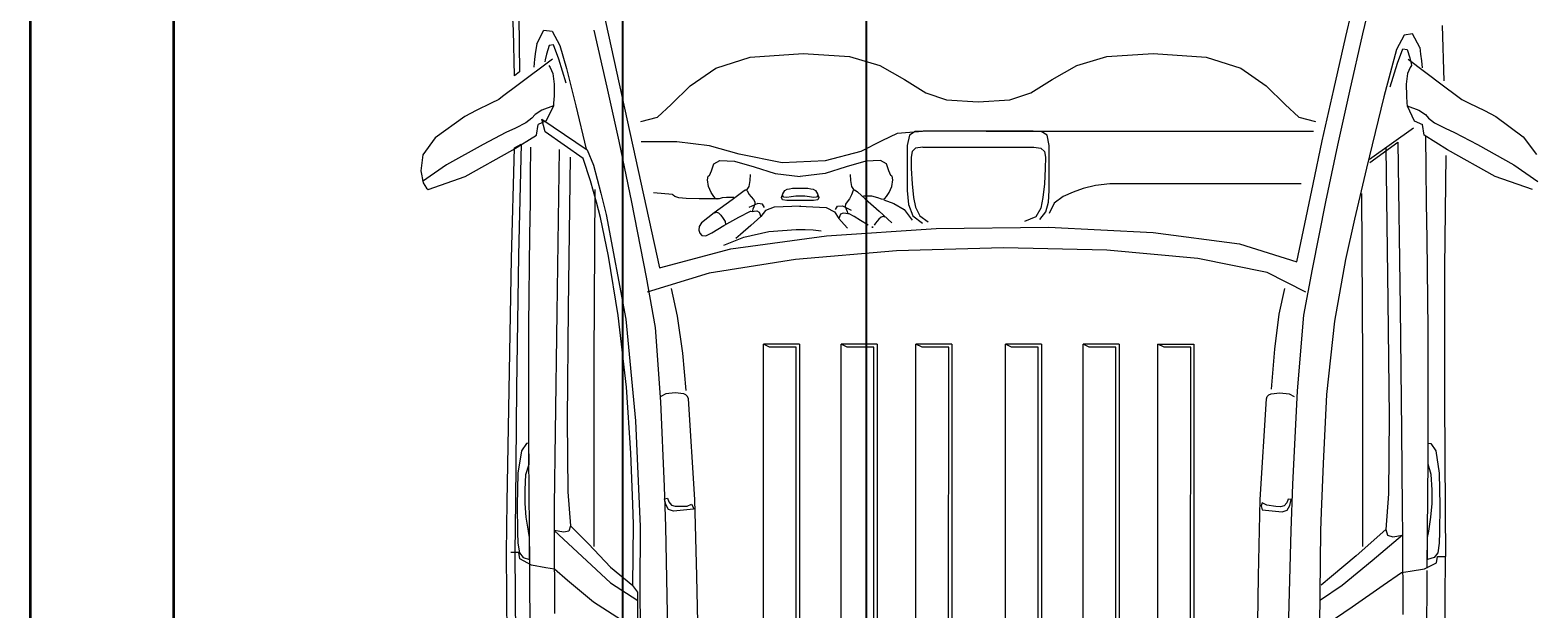
# Model space of a CAD drawing. Units: inches. Extents: x 5 to 421, y -617 to 43.
# Tile 3 of 15: x 37 to 132, y -505 to -469. Entities that reach past the tile are written whole.
import ezdxf

# ---------------------------------------------------------------- set-up
doc = ezdxf.new("R2010")
doc.units = ezdxf.units.IN
doc.header["$MEASUREMENT"] = 0
for name, color, linetype, lineweight in [('A-ANNO-DIMS', 2, 'Continuous', 18), ('A-SITE-VEHC', 8, 'Continuous', 13), ('A-WALL', 7, 'Continuous', 35)]:
    doc.layers.add(name, color=color, linetype=linetype, lineweight=lineweight)
doc.styles.get("Standard").update_dxf_attribs({"font": 'arial.ttf'})
doc.dimstyles.get("Standard").update_dxf_attribs({"dimtxt": 0.18, "dimasz": 0.18, "dimexe": 0.18, "dimexo": 0.0625, "dimgap": 0.09, "dimtad": 0, "dimtih": 1, "dimtoh": 1, "dimdec": 0, "dimzin": 0, "dimdsep": 46, "dimlunit": 3, "dimtxsty": 'Standard', "dimcen": 0.09, "dimadec": 0, "dimazin": 0, "dimtfac": 1, "dimtdec": 0, "dimtofl": 0, "dimtmove": 0, "dimatfit": 3, "dimfxl": 1, "dimtolj": 1, "dimtzin": 0, "dimarcsym": 0})

# ---------------------------------------------------------------- blocks, each defined once
blk = doc.blocks.new('*D78')
at = {"layer": 'A-ANNO-DIMS', "color": 0, "lineweight": -2, "transparency": 16777216}
for p, q in [((74.624, -338.19), (74.624, -616.599)), ((89.924, -338.331), (89.924, -616.599)), ((74.804, -616.419), (81.958, -616.419)), ((89.744, -616.419), (82.589, -616.419))]:
    blk.add_line(p, q, dxfattribs=at)
at = {"layer": 'A-ANNO-DIMS', "color": 0, "transparency": 16777216}
for points in [[(74.804, -616.389), (74.804, -616.449), (74.624, -616.419)], [(89.744, -616.389), (89.744, -616.449), (89.924, -616.419)]]:
    blk.add_solid(points, dxfattribs=at)
at = {"layer": 'Defpoints', "color": 0, "transparency": 16777216}
for p in [(74.624, -338.127), (89.924, -338.269), (89.924, -616.419)]:
    blk.add_point(p, dxfattribs=at)
at = {"layer": 'A-ANNO-DIMS', "color": 0, "transparency": 16777216, "insert": (82.274, -616.419), "char_height": 0.18, "attachment_point": 5}
blk.add_mtext('\\A1;15.3', dxfattribs=at)

msp = doc.modelspace()

# ---------------------------------------------------------------- linework, layer by layer
at = {"layer": 'A-SITE-VEHC'}
for p, q in [((67.7642, -468.9053), (67.6725, -466.951)), ((73.4116, -467.6765), (76.9484, -483.8294)), ((121.4807, -467.4597), (121.0957, -469.1284)), ((68.1156, -468.0292), (68.1428, -471.5036)), ((120.0545, -469.2979), (120.4101, -467.7799)), ((126.0856, -468.6013), (126.1926, -472.0787)), ((67.8382, -471.7647), (67.7642, -468.9053)), ((69.2294, -469.7473), (69.6829, -468.8901)), ((69.6829, -468.8901), (70.1988, -468.9567)), ((70.1988, -468.9567), (70.69, -469.8597)), ((72.8166, -468.888), (73.6384, -472.4794)), ((119.2871, -472.6093), (120.0545, -469.2979)), ((121.0957, -469.1284), (120.2738, -472.7197)), ((123.7131, -469.197), (123.2221, -470.1)), ((124.2292, -469.1304), (123.7131, -469.197)), ((124.6827, -469.9876), (124.2292, -469.1304)), ((69.1614, -470.2267), (69.1022, -470.7152)), ((69.2294, -469.7473), (69.1614, -470.2267)), ((69.843, -470.3966), (69.7577, -470.7462)), ((70.0157, -469.8597), (69.843, -470.3966)), ((70.28, -469.8223), (70.0157, -469.8597)), ((70.6316, -470.7212), (70.28, -469.8223)), ((70.69, -469.8597), (71.0943, -471.2901)), ((82.6431, -470.5843), (85.9655, -470.3515)), ((85.9655, -470.3515), (88.8787, -470.5475)), ((88.8787, -470.5475), (90.7773, -471.1094)), ((103.1439, -471.1094), (105.0426, -470.5475)), ((105.0426, -470.5475), (107.9558, -470.3515)), ((107.9558, -470.3515), (111.2783, -470.5843)), ((123.2221, -470.1), (122.4253, -473.0796)), ((123.2804, -470.9615), (123.632, -470.0626)), ((123.632, -470.0626), (123.8964, -470.1)), ((123.8964, -470.1), (124.069, -470.6368)), ((124.6827, -469.9876), (124.7423, -470.4038)), ((124.7423, -470.4038), (124.7953, -470.8268)), ((68.1428, -471.5036), (67.8382, -471.7647)), ((70.2201, -470.718), (68.0729, -472.3222)), ((69.1022, -470.7152), (69.0508, -471.213)), ((69.7577, -470.7462), (69.7349, -470.8711)), ((69.9956, -471.1111), (70.083, -471.2298)), ((70.083, -471.2298), (70.2453, -471.6105)), ((71.0831, -472.2194), (70.6316, -470.7212)), ((71.0943, -471.2901), (71.6877, -473.6545)), ((78.8717, -472.3887), (80.4797, -471.2698)), ((80.4797, -471.2698), (82.6431, -470.5843)), ((90.7773, -471.1094), (92.3227, -471.9987)), ((101.5986, -471.9987), (103.1439, -471.1094)), ((111.2783, -470.5843), (113.4418, -471.2698)), ((113.4418, -471.2698), (115.0496, -472.3887)), ((122.8289, -472.4594), (123.2804, -470.9615)), ((124.0898, -471.2298), (123.9277, -471.6105)), ((123.9524, -470.718), (126.0997, -472.3222)), ((124.069, -470.6368), (124.1543, -470.9863)), ((124.1771, -471.1111), (124.0898, -471.2298)), ((124.1543, -470.9863), (124.1771, -471.1111)), ((124.7953, -470.8268), (124.8422, -471.2569)), ((68.0729, -472.3222), (67.0866, -473.065)), ((70.2453, -471.6105), (70.3327, -472.291)), ((70.3327, -472.291), (70.3182, -473.015)), ((77.6783, -473.5667), (78.8717, -472.3887)), ((92.3227, -471.9987), (93.6601, -472.8207)), ((100.2614, -472.8207), (101.5986, -471.9987)), ((115.0496, -472.3887), (116.2431, -473.5667)), ((123.9277, -471.6105), (123.8403, -472.291)), ((123.8403, -472.291), (123.8549, -473.015)), ((126.0997, -472.3222), (127.086, -473.065)), ((66.8494, -473.2461), (66.373, -473.4764)), ((67.0866, -473.065), (66.8494, -473.2461)), ((70.3182, -473.015), (70.291, -473.4769)), ((73.6384, -472.4794), (74.3978, -475.8708)), ((93.6601, -472.8207), (94.9685, -473.2574)), ((94.9685, -473.2574), (96.9608, -473.3858)), ((96.9608, -473.3858), (98.953, -473.2574)), ((98.953, -473.2574), (100.2614, -472.8207)), ((118.5569, -475.8501), (119.2871, -472.6093)), ((120.2738, -472.7197), (119.5142, -476.1112)), ((122.4253, -473.0796), (121.3413, -477.5698)), ((123.8549, -473.015), (123.8818, -473.4769)), ((127.086, -473.065), (127.3231, -473.2461)), ((127.3231, -473.2461), (127.7999, -473.4756)), ((64.7148, -474.3134), (62.8626, -475.6479)), ((65.4224, -473.9441), (64.7148, -474.3134)), ((66.373, -473.4764), (65.4224, -473.9441)), ((69.1278, -474.1845), (68.9282, -474.4258)), ((69.5523, -473.9181), (69.1278, -474.1845)), ((70.2764, -473.6392), (69.5523, -473.9181)), ((70.2764, -473.6392), (69.8269, -474.5943)), ((70.291, -473.4769), (70.2764, -473.6392)), ((71.6877, -473.6545), (72.3416, -476.3662)), ((75.7798, -474.6283), (76.8189, -474.356)), ((76.8189, -474.356), (77.6783, -473.5667)), ((116.2431, -473.5667), (117.1025, -474.356)), ((117.1025, -474.356), (118.1418, -474.6283)), ((123.8818, -473.4769), (123.8964, -473.6392)), ((123.8964, -473.6392), (124.3459, -474.5943)), ((123.8964, -473.6392), (124.6203, -473.9181)), ((124.6203, -473.9181), (125.0448, -474.1845)), ((125.0448, -474.1845), (125.2446, -474.4258)), ((127.7999, -473.4756), (128.7512, -473.9425)), ((128.7512, -473.9425), (129.458, -474.3134)), ((129.458, -474.3134), (131.1824, -475.5849)), ((67.8961, -475.0418), (67.2989, -475.3245)), ((68.5557, -474.7088), (67.8961, -475.0418)), ((68.9282, -474.4258), (68.5557, -474.7088)), ((69.209, -475.4933), (69.3213, -474.819)), ((69.8269, -474.5943), (69.3213, -474.819)), ((69.5573, -474.4845), (72.4075, -476.3993)), ((69.753, -475.2679), (69.5573, -474.4845)), ((72.1464, -476.9434), (69.753, -475.2679)), ((93.732, -475.2351), (91.865, -475.3861)), ((93.0014, -475.264), (92.6364, -475.4898)), ((93.5076, -475.2374), (93.0014, -475.264)), ((100.414, -475.2374), (93.5076, -475.2374)), ((97.4687, -475.2546), (93.732, -475.2351)), ((103.1448, -475.2665), (97.4687, -475.2546)), ((100.9201, -475.264), (100.414, -475.2374)), ((101.2849, -475.4898), (100.9201, -475.264)), ((110.1834, -475.2654), (103.1448, -475.2665)), ((118.0075, -475.2463), (110.1834, -475.2654)), ((124.2895, -475.0438), (121.5368, -477.0099)), ((124.3459, -474.5943), (124.8514, -474.819)), ((124.9638, -475.4933), (124.8514, -474.819)), ((125.2446, -474.4258), (125.617, -474.7088)), ((125.617, -474.7088), (126.2767, -475.0418)), ((126.2767, -475.0418), (126.874, -475.3245)), ((62.8626, -475.6479), (62.0839, -476.7266)), ((65.8678, -476.071), (63.574, -477.3502)), ((67.2989, -475.3245), (65.8678, -476.071)), ((67.7321, -476.4144), (69.209, -475.4933)), ((67.8382, -476.2907), (68.2514, -476.0431)), ((68.2514, -476.0431), (68.0884, -483.0214)), ((68.8353, -476.2417), (68.8173, -478.0422)), ((74.3978, -475.8708), (75.191, -479.7057)), ((78.036, -475.8989), (75.7823, -475.8989)), ((80.0909, -476.16), (78.036, -475.8989)), ((81.9383, -476.6824), (80.0909, -476.16)), ((90.9118, -475.8357), (89.5976, -476.5082)), ((91.865, -475.3861), (90.9118, -475.8357)), ((92.6364, -475.4898), (92.4962, -476.1328)), ((92.4962, -476.1328), (92.4962, -478.9649)), ((93.4786, -476.2485), (93.0243, -476.3068)), ((93.4786, -476.2485), (100.4427, -476.2485)), ((100.4427, -476.2485), (100.897, -476.3068)), ((101.4251, -476.1328), (101.2849, -475.4898)), ((101.4251, -478.9649), (101.4251, -476.1328)), ((117.9842, -478.5661), (118.5569, -475.8501)), ((119.5142, -476.1112), (118.7684, -479.682)), ((121.5478, -477.2038), (123.309, -475.9301)), ((123.309, -475.9301), (123.4489, -486.3059)), ((126.4406, -476.4144), (124.9638, -475.4933)), ((125.0558, -475.5226), (125.0783, -477.5679)), ((126.874, -475.3245), (128.3048, -476.071)), ((128.3048, -476.071), (130.5986, -477.3502)), ((131.1824, -475.5849), (132.0249, -476.6951)), ((62.0839, -476.7266), (61.9559, -477.7221)), ((64.7434, -478.0929), (67.7321, -476.4144)), ((67.6582, -483.2319), (67.8382, -476.2907)), ((70.6419, -476.3828), (70.4967, -486.6394)), ((71.3384, -476.86), (71.2002, -486.3499)), ((72.6059, -478.3474), (72.1464, -476.9434)), ((72.4075, -476.3993), (72.7889, -477.3696)), ((80.3474, -477.2968), (80.7381, -477.069)), ((80.7381, -477.069), (81.6458, -477.1299)), ((81.6458, -477.1299), (82.8903, -477.4798)), ((84.6376, -477.2251), (81.9383, -476.6824)), ((87.3448, -477.0939), (84.6376, -477.2251)), ((89.5976, -476.5082), (87.3448, -477.0939)), ((89.9099, -477.1299), (88.6653, -477.4798)), ((90.8176, -477.069), (89.9099, -477.1299)), ((91.2083, -477.2968), (90.8176, -477.069)), ((92.8013, -476.5032), (92.742, -476.8699)), ((92.742, -476.8699), (92.7575, -477.5831)), ((93.0243, -476.3068), (92.8013, -476.5032)), ((100.897, -476.3068), (101.1202, -476.5032)), ((101.1202, -476.5032), (101.1796, -476.8699)), ((101.1796, -476.8699), (101.1641, -477.5831)), ((122.5482, -476.2796), (122.6903, -485.8978)), ((126.3277, -476.7692), (126.2495, -483.7891)), ((129.4293, -478.0929), (126.4406, -476.4144)), ((61.9559, -477.7221), (62.0973, -478.4772)), ((63.574, -477.3502), (62.068, -478.3964)), ((62.4051, -478.9016), (64.7434, -478.0929)), ((68.8173, -478.0422), (68.8113, -479.7258)), ((72.7889, -477.3696), (73.2598, -479.1349)), ((79.9553, -478.2858), (80.0062, -478.06)), ((80.0062, -478.06), (80.0922, -478.0108)), ((80.0922, -478.0108), (80.2008, -477.7367)), ((80.2008, -477.7367), (80.3474, -477.2968)), ((82.6282, -477.9535), (82.6122, -478.3426)), ((82.8903, -477.4798), (84.2152, -477.8876)), ((84.2152, -477.8876), (85.778, -478.0834)), ((87.3403, -477.8876), (85.778, -478.0834)), ((88.6653, -477.4798), (87.3403, -477.8876)), ((88.9275, -477.9535), (88.9463, -478.3409)), ((91.3549, -477.7367), (91.2083, -477.2968)), ((91.4635, -478.0108), (91.3549, -477.7367)), ((91.5496, -478.06), (91.4635, -478.0108)), ((91.6004, -478.2858), (91.5496, -478.06)), ((92.7575, -477.5831), (92.8083, -478.55)), ((101.1641, -477.5831), (101.1133, -478.55)), ((121.3413, -477.5698), (120.5817, -480.7741)), ((125.0783, -477.5679), (125.0952, -479.7298)), ((131.7676, -478.9016), (129.4293, -478.0929)), ((130.5986, -477.3502), (132.1045, -478.3964)), ((62.0973, -478.4772), (62.3011, -478.8205)), ((62.3011, -478.8205), (62.4051, -478.9016)), ((72.989, -479.703), (72.6059, -478.3474)), ((72.8809, -478.9048), (72.8154, -489.5141)), ((80.0217, -478.7197), (79.9553, -478.2858)), ((80.1972, -479.0895), (80.0217, -478.7197)), ((80.3599, -479.3406), (80.1972, -479.0895)), ((82.1803, -479.0372), (81.4976, -479.5399)), ((82.3213, -478.9449), (82.1803, -479.0372)), ((82.377, -478.9445), (82.3213, -478.9449)), ((82.3869, -478.9611), (82.377, -478.9445)), ((82.5525, -478.7149), (82.3869, -478.9611)), ((82.4445, -478.9643), (82.5487, -479.1852)), ((82.6122, -478.3426), (82.5525, -478.7149)), ((84.68, -479.1671), (84.8179, -478.9691)), ((84.8179, -478.9691), (84.9656, -478.8835)), ((84.9656, -478.8835), (85.1133, -478.8494)), ((85.1133, -478.8494), (85.2952, -478.8253)), ((85.2952, -478.8253), (85.5285, -478.8109)), ((85.5285, -478.8109), (85.778, -478.806)), ((85.778, -478.806), (86.0272, -478.8109)), ((86.0272, -478.8109), (86.2605, -478.8253)), ((86.2605, -478.8253), (86.4424, -478.8494)), ((86.4424, -478.8494), (86.5902, -478.8835)), ((86.5902, -478.8835), (86.7378, -478.9691)), ((86.7378, -478.9691), (86.876, -479.1671)), ((88.9463, -478.3409), (89.01, -478.7123)), ((89.1153, -478.9649), (89.0078, -479.2255)), ((89.01, -478.7123), (89.1732, -478.9649)), ((89.1732, -478.9649), (89.1839, -478.9488)), ((89.1839, -478.9488), (89.2395, -478.952)), ((89.2395, -478.952), (89.3754, -479.0515)), ((89.3754, -479.0515), (89.8697, -479.4918)), ((91.1957, -479.3406), (91.3586, -479.0895)), ((91.3586, -479.0895), (91.5341, -478.7197)), ((91.5341, -478.7197), (91.6004, -478.2858)), ((92.4962, -478.9649), (92.5716, -479.8398)), ((92.8083, -478.55), (92.9009, -479.3982)), ((101.1133, -478.55), (101.0207, -479.3982)), ((101.3768, -479.6895), (101.4251, -478.9649)), ((102.9143, -479.0757), (102.3026, -479.3378)), ((103.5512, -478.8437), (102.9143, -479.0757)), ((104.3232, -478.6407), (103.5512, -478.8437)), ((105.2211, -478.5536), (104.3232, -478.6407)), ((117.2322, -478.5536), (105.2211, -478.5536)), ((117.3032, -481.8491), (117.9842, -478.5661)), ((68.8113, -479.7258), (68.7799, -481.7696)), ((73.2345, -480.6643), (72.989, -479.703)), ((73.2598, -479.1349), (73.5841, -480.4723)), ((75.191, -479.7057), (76.1125, -484.4179)), ((77.7606, -479.2065), (76.5655, -479.1193)), ((77.7944, -479.2533), (77.7606, -479.2065)), ((77.9152, -479.3482), (77.7944, -479.2533)), ((78.1522, -479.424), (77.9152, -479.3482)), ((78.6137, -479.4592), (78.1522, -479.424)), ((79.4366, -479.4787), (78.6137, -479.4592)), ((80.692, -479.4848), (79.4366, -479.4787)), ((80.4653, -479.4678), (80.3599, -479.3406)), ((81.4976, -479.5399), (80.3707, -480.3697)), ((80.5673, -479.5116), (80.4653, -479.4678)), ((80.692, -479.4848), (80.5673, -479.5116)), ((80.8702, -479.4277), (80.692, -479.4848)), ((81.1545, -479.3929), (80.8702, -479.4277)), ((81.6024, -479.4128), (81.1545, -479.3929)), ((82.5487, -479.1852), (82.6908, -479.3628)), ((83.1232, -479.7795), (82.5499, -480.0244)), ((82.6908, -479.3628), (82.8367, -479.5185)), ((82.8705, -479.9834), (82.8052, -480.1348)), ((82.8367, -479.5185), (82.9275, -479.6658)), ((82.9348, -479.8152), (82.8705, -479.9834)), ((82.9275, -479.6658), (82.9348, -479.8152)), ((83.418, -479.8191), (83.1232, -479.7795)), ((83.5333, -480.0327), (83.418, -479.8191)), ((84.1398, -480.0095), (83.603, -480.2164)), ((85.8213, -479.9474), (84.1398, -480.0095)), ((84.6028, -479.4014), (84.68, -479.1671)), ((84.6702, -479.549), (84.6028, -479.4014)), ((84.9398, -479.6003), (84.6702, -479.549)), ((84.6703, -479.2854), (84.68, -479.1671)), ((84.7569, -479.3909), (84.6703, -479.2854)), ((84.9398, -479.4128), (84.7569, -479.3909)), ((85.2027, -479.3672), (84.9398, -479.4128)), ((86.6159, -479.6003), (84.9398, -479.6003)), ((85.5008, -479.3282), (85.2027, -479.3672)), ((85.7923, -479.3116), (85.5008, -479.3282)), ((85.7344, -479.9474), (87.409, -480.0372)), ((86.0764, -479.3282), (85.7923, -479.3116)), ((86.3607, -479.3672), (86.0764, -479.3282)), ((86.6159, -479.4128), (86.3607, -479.3672)), ((86.7989, -479.3909), (86.6159, -479.4128)), ((86.8855, -479.549), (86.6159, -479.6003)), ((86.8855, -479.2854), (86.7989, -479.3909)), ((86.876, -479.1671), (86.953, -479.4014)), ((86.876, -479.1671), (86.8855, -479.2854)), ((86.953, -479.4014), (86.8855, -479.549)), ((87.409, -480.0372), (87.9274, -480.3005)), ((88.003, -480.1495), (88.1293, -479.9425)), ((88.1293, -479.9425), (88.4257, -479.9184)), ((88.4257, -479.9184), (88.9854, -480.1928)), ((88.6268, -479.8151), (88.6118, -479.9639)), ((88.6118, -479.9639), (88.6673, -480.1352)), ((88.7253, -479.6729), (88.6268, -479.8151)), ((88.8714, -479.4797), (88.7253, -479.6729)), ((89.0078, -479.2255), (88.8714, -479.4797)), ((89.751, -479.2973), (90.2515, -479.3074)), ((89.8697, -479.4918), (90.733, -480.2632)), ((90.2515, -479.3074), (90.633, -479.3977)), ((90.633, -479.3977), (90.8637, -479.4848)), ((90.8637, -479.4848), (90.9883, -479.5116)), ((90.9883, -479.5116), (91.0904, -479.4678)), ((91.0337, -479.5545), (91.6608, -479.7849)), ((91.0904, -479.4678), (91.1957, -479.3406)), ((91.6608, -479.7849), (92.3072, -480.1508)), ((92.5716, -479.8398), (92.8607, -480.5492)), ((92.9009, -479.3982), (93.03, -480.0061)), ((93.03, -480.0061), (93.2956, -480.5618)), ((101.0207, -479.3982), (100.8845, -480.0651)), ((101.1974, -480.3106), (101.3768, -479.6895)), ((101.7345, -479.7496), (101.413, -480.4032)), ((102.3026, -479.3378), (101.7345, -479.7496)), ((118.7684, -479.682), (117.9259, -483.9027)), ((121.0312, -479.1448), (121.0957, -489.692)), ((125.0952, -479.7298), (125.1322, -482.01)), ((73.7374, -483.0953), (73.2345, -480.6643)), ((73.5841, -480.4723), (74.822, -487.0365)), ((79.5908, -480.9979), (79.4373, -481.2261)), ((80.3707, -480.3697), (79.5908, -480.9979)), ((80.4198, -480.3612), (80.532, -480.3302)), ((80.532, -480.3302), (80.6469, -480.3668)), ((80.6469, -480.3668), (80.7882, -480.5108)), ((80.7882, -480.5108), (80.9472, -480.7169)), ((80.9472, -480.7169), (81.0651, -480.9112)), ((80.9758, -481.1711), (81.9336, -480.6389)), ((81.0651, -480.9112), (81.0906, -481.0909)), ((81.9336, -480.6389), (82.6677, -480.2622)), ((82.6677, -480.2622), (82.6882, -480.2691)), ((83.3009, -480.5991), (82.6773, -481.1681)), ((82.6882, -480.2691), (82.7569, -480.2753)), ((82.7569, -480.2753), (82.8848, -480.259)), ((82.7849, -480.2243), (82.7839, -480.2536)), ((82.8052, -480.1348), (82.7849, -480.2243)), ((82.8848, -480.259), (83.0529, -480.241)), ((83.0529, -480.241), (83.2062, -480.3219)), ((83.2062, -480.3219), (83.3009, -480.5991)), ((83.603, -480.2164), (83.3009, -480.5991)), ((87.9274, -480.3005), (88.2051, -480.7276)), ((88.3143, -480.4558), (88.2051, -480.7276)), ((88.2051, -480.7276), (88.3742, -480.9137)), ((88.4716, -480.3829), (88.3143, -480.4558)), ((88.3742, -480.9137), (88.5481, -481.1049)), ((88.6387, -480.4096), (88.4716, -480.3829)), ((88.7654, -480.4326), (88.6387, -480.4096)), ((88.6673, -480.1352), (88.7247, -480.2898)), ((88.7247, -480.2898), (88.7402, -480.3802)), ((88.7402, -480.3802), (88.7396, -480.4096)), ((88.8344, -480.4298), (88.7654, -480.4326)), ((88.8552, -480.4239), (88.8344, -480.4298)), ((89.1642, -480.5964), (88.8552, -480.4239)), ((89.5751, -480.8394), (89.1642, -480.5964)), ((90.0561, -481.1364), (89.5751, -480.8394)), ((90.6105, -480.8958), (90.5108, -481.017)), ((90.7192, -480.771), (90.6105, -480.8958)), ((90.868, -480.6344), (90.7192, -480.771)), ((90.733, -480.2632), (91.5256, -480.9935)), ((90.9846, -480.6039), (90.868, -480.6344)), ((91.0948, -480.6407), (90.9846, -480.6039)), ((92.3072, -480.1508), (92.8181, -480.8165)), ((92.8607, -480.5492), (93.4586, -481.0195)), ((93.2956, -480.5618), (93.8219, -480.9285)), ((100.5682, -480.6266), (99.8639, -480.9177)), ((100.8845, -480.0651), (100.5682, -480.6266)), ((100.8352, -480.7866), (101.1974, -480.3106)), ((120.5817, -480.7741), (120.0178, -483.2917)), ((68.7799, -481.7696), (68.7153, -487.4645)), ((79.4373, -481.2261), (79.4049, -481.4462)), ((79.4049, -481.4462), (79.4701, -481.6426)), ((79.4701, -481.6426), (79.6096, -481.7925)), ((79.6096, -481.7925), (79.8488, -481.8189)), ((79.8488, -481.8189), (80.2377, -481.6248)), ((80.2377, -481.6248), (80.9758, -481.1711)), ((80.9839, -482.3955), (82.2434, -481.8945)), ((81.4275, -482.6347), (87.4383, -481.8043)), ((82.0306, -481.7213), (81.7324, -481.9698)), ((82.6773, -481.1681), (82.0306, -481.7213)), ((82.2434, -481.8945), (83.801, -481.5405)), ((83.801, -481.5405), (85.5322, -481.4064)), ((85.5322, -481.4064), (86.0915, -481.4083)), ((86.0915, -481.4083), (86.5861, -481.4286)), ((86.5861, -481.4286), (87.1058, -481.4885)), ((87.4383, -481.8043), (94.3095, -481.3477)), ((88.5481, -481.1049), (88.7556, -481.3296)), ((90.2862, -481.273), (90.368, -481.267)), ((90.3134, -481.271), (90.2862, -481.273)), ((90.3407, -481.2689), (90.3134, -481.271)), ((90.368, -481.267), (90.3407, -481.2689)), ((90.5108, -481.017), (90.433, -481.1345)), ((94.3095, -481.3477), (101.3698, -481.274)), ((101.3698, -481.274), (107.9483, -481.5928)), ((107.9483, -481.5928), (113.3734, -482.3131)), ((116.974, -483.4445), (117.3032, -481.8491)), ((76.9484, -483.8294), (81.4275, -482.6347)), ((91.8309, -482.7563), (85.4835, -483.2928)), ((98.5386, -482.5616), (91.8309, -482.7563)), ((105.0343, -482.7165), (98.5386, -482.5616)), ((110.7459, -483.2291), (105.0343, -482.7165)), ((113.3734, -482.3131), (116.974, -483.4445)), ((125.1322, -482.01), (125.1968, -487.7049)), ((67.499, -491.4989), (67.6582, -483.2319)), ((68.0884, -483.0214), (67.9667, -491.3737)), ((74.3419, -486.814), (73.7374, -483.0953)), ((85.4835, -483.2928), (80.0686, -484.163)), ((115.1011, -484.1073), (110.7459, -483.2291)), ((120.0178, -483.2917), (119.3291, -487.1701)), ((126.2495, -483.7891), (126.2526, -492.1035)), ((76.1125, -484.4179), (76.661, -487.5713)), ((80.0686, -484.163), (76.1583, -485.3591)), ((117.5277, -485.3591), (115.1011, -484.1073)), ((117.9259, -483.9027), (117.3946, -486.7878)), ((77.6734, -485.1251), (78.0555, -486.8513)), ((116.1976, -485.1251), (115.8454, -486.7417)), ((70.4967, -486.6394), (70.3961, -494.1413)), ((71.2002, -486.3499), (71.1405, -493.3527)), ((122.6903, -485.8978), (122.7588, -493.1827)), ((123.4489, -486.3059), (123.5378, -494.0695)), ((68.7153, -487.4645), (68.7134, -493.0971)), ((74.8664, -491.3266), (74.3419, -486.814)), ((74.822, -487.0365), (75.4434, -493.4318)), ((76.661, -487.5713), (77.0103, -492.2485)), ((78.0555, -486.8513), (78.3795, -489.1723)), ((115.8454, -486.7417), (115.5683, -488.9337)), ((117.3946, -486.7878), (116.9945, -491.5463)), ((119.3291, -487.1701), (118.8403, -491.785)), ((125.1968, -487.7049), (125.1989, -493.3375)), ((72.8154, -489.5141), (72.8116, -497.9174)), ((78.3795, -489.1723), (78.5874, -491.522)), ((83.8564, -488.8077), (83.4721, -488.6203)), ((85.7372, -488.6203), (83.4721, -488.6203)), ((83.4744, -547.9801), (83.4744, -488.6203)), ((85.5319, -488.8077), (83.8564, -488.8077)), ((85.5102, -547.0362), (85.5319, -488.8077)), ((85.7354, -488.6203), (85.7354, -547.9801)), ((85.7372, -488.6203), (85.7372, -547.9801)), ((88.7307, -488.8077), (88.3465, -488.6203)), ((90.6116, -488.6203), (88.3465, -488.6203)), ((88.3484, -547.9801), (88.3484, -488.6203)), ((90.4059, -488.8077), (88.7307, -488.8077)), ((90.3843, -547.0362), (90.4059, -488.8077)), ((90.6093, -488.6203), (90.6093, -547.9801)), ((90.6116, -488.6203), (90.6116, -547.9801)), ((93.4306, -488.8077), (93.0463, -488.6203)), ((95.3114, -488.6203), (93.0463, -488.6203)), ((93.0486, -547.9801), (93.0486, -488.6203)), ((95.106, -488.8077), (93.4306, -488.8077)), ((95.0844, -547.0362), (95.106, -488.8077)), ((95.3095, -488.6203), (95.3095, -547.9801)), ((95.3114, -488.6203), (95.3114, -547.9801)), ((99.0539, -488.8077), (98.6697, -488.6203)), ((100.9348, -488.6203), (98.6697, -488.6203)), ((98.6716, -547.9801), (98.6716, -488.6203)), ((100.7295, -488.8077), (99.0539, -488.8077)), ((100.7075, -547.0362), (100.7295, -488.8077)), ((100.9326, -488.6203), (100.9326, -547.9801)), ((100.9348, -488.6203), (100.9348, -547.9801)), ((103.928, -488.8077), (103.544, -488.6203)), ((105.8088, -488.6203), (103.544, -488.6203)), ((103.5459, -547.9801), (103.5459, -488.6203)), ((105.6034, -488.8077), (103.928, -488.8077)), ((105.5818, -547.0362), (105.6034, -488.8077)), ((105.8069, -488.6203), (105.8069, -547.9801)), ((105.8088, -488.6203), (105.8088, -547.9801)), ((108.2458, -547.9801), (108.2458, -488.6203)), ((108.6301, -488.8077), (108.2458, -488.6203)), ((108.2458, -488.6203), (110.509, -488.6203)), ((110.3055, -488.8077), (108.6301, -488.8077)), ((110.2835, -547.0362), (110.3055, -488.8077)), ((110.509, -488.6203), (110.509, -547.9801)), ((115.5683, -488.9337), (115.361, -491.4352)), ((121.0957, -489.692), (121.0979, -497.9794)), ((67.9667, -491.3737), (67.8899, -498.4751)), ((75.1489, -495.4585), (74.8664, -491.3266)), ((67.3847, -498.5143), (67.499, -491.4989)), ((77.0103, -492.2485), (77.2378, -497.5567)), ((77.3306, -491.7401), (77.0191, -491.9143)), ((77.9255, -491.6749), (77.3306, -491.7401)), ((78.4632, -491.7268), (77.9255, -491.6749)), ((78.6011, -491.7951), (78.4632, -491.7268)), ((78.7119, -491.9076), (78.6011, -491.7951)), ((78.7615, -492.0445), (78.7119, -491.9076)), ((79.1687, -498.3726), (78.7615, -492.0445)), ((114.6627, -498.3726), (115.0563, -492.0445)), ((115.0563, -492.0445), (115.1059, -491.9076)), ((115.1059, -491.9076), (115.2166, -491.7951)), ((115.2166, -491.7951), (115.3543, -491.7268)), ((115.3543, -491.7268), (115.8921, -491.6749)), ((115.8921, -491.6749), (116.4871, -491.7401)), ((116.4871, -491.7401), (116.7987, -491.9143)), ((116.9945, -491.5463), (116.7047, -497.4395)), ((118.8403, -491.785), (118.6134, -496.1213)), ((126.2526, -492.1035), (126.2892, -499.0468)), ((68.7134, -493.0971), (68.7238, -495.646)), ((122.7588, -493.1827), (122.7219, -498.0132)), ((70.3961, -494.1413), (70.3377, -498.7465)), ((71.1405, -493.3527), (71.1862, -497.901)), ((75.4434, -493.4318), (75.7263, -500.0787)), ((123.5378, -494.0695), (123.5847, -498.9363)), ((125.1989, -493.3375), (125.1886, -495.8864)), ((68.5864, -494.8629), (68.2725, -495.3175)), ((68.7461, -494.8307), (68.5864, -494.8629)), ((68.7588, -496.1557), (68.7461, -494.8307)), ((125.208, -496.1557), (125.2207, -494.8307)), ((125.2207, -494.8307), (125.3804, -494.8629)), ((125.3804, -494.8629), (125.6942, -495.3175)), ((68.2725, -495.3175), (68.0521, -496.731)), ((68.7238, -495.646), (68.7799, -502.4435)), ((75.2736, -498.6582), (75.1489, -495.4585)), ((118.6134, -496.1213), (118.4864, -499.1718)), ((125.1886, -495.8864), (125.1322, -502.6839)), ((125.6942, -495.3175), (125.9147, -496.731)), ((68.0521, -496.731), (68.0138, -498.7612)), ((68.5045, -497.7663), (68.5587, -496.8064)), ((68.5587, -496.8064), (68.7588, -496.1557)), ((125.408, -496.8064), (125.208, -496.1557)), ((125.4623, -497.7663), (125.408, -496.8064)), ((125.9147, -496.731), (125.9529, -498.7612)), ((68.5064, -498.6312), (68.5045, -497.7663)), ((71.1862, -497.901), (71.3639, -500.0278)), ((72.8116, -497.9174), (72.821, -501.336)), ((77.2378, -497.5567), (77.319, -500.0842)), ((116.7047, -497.4395), (116.593, -500.3246)), ((121.0979, -497.9794), (121.0876, -501.3357)), ((122.7219, -498.0132), (122.5482, -500.2682)), ((125.4604, -498.6312), (125.4623, -497.7663)), ((67.339, -501.7004), (67.3847, -498.5143)), ((67.8899, -498.4751), (67.8614, -501.7001)), ((68.0138, -498.7612), (68.0355, -500.4285)), ((68.5794, -499.4863), (68.5064, -498.6312)), ((70.3377, -498.7465), (70.3187, -500.3131)), ((75.3016, -499.9431), (75.2736, -498.6582)), ((77.2602, -498.3405), (77.4543, -498.3004)), ((77.3508, -498.6987), (77.2602, -498.3405)), ((77.5176, -499.0018), (77.3508, -498.6987)), ((77.4543, -498.3004), (77.5364, -498.5311)), ((77.5364, -498.5311), (77.6924, -498.7234)), ((77.6924, -498.7234), (77.9236, -498.7862)), ((79.0766, -498.9836), (77.8131, -499.1078)), ((77.9236, -498.7862), (78.1912, -498.7995)), ((78.1912, -498.7995), (78.6865, -498.7874)), ((78.6865, -498.7874), (78.9484, -498.6717)), ((78.9484, -498.6717), (79.0471, -498.818)), ((79.0471, -498.818), (79.0762, -498.9355)), ((79.0762, -498.9355), (79.0766, -498.9836)), ((79.2954, -503.1925), (79.1687, -498.3726)), ((114.5618, -503.1925), (114.6627, -498.3726)), ((114.7921, -498.5847), (114.7271, -498.7647)), ((114.7271, -498.7647), (114.761, -498.945)), ((114.761, -498.945), (114.7943, -499.0269)), ((115.0875, -498.7343), (114.7921, -498.5847)), ((115.6456, -498.8093), (115.0875, -498.7343)), ((115.9471, -498.8298), (115.6456, -498.8093)), ((116.1785, -498.767), (115.9471, -498.8298)), ((116.3346, -498.5748), (116.1785, -498.767)), ((116.4167, -498.3441), (116.3346, -498.5748)), ((116.3534, -499.0454), (116.5202, -498.7421)), ((116.6108, -498.3842), (116.4167, -498.3441)), ((116.5202, -498.7421), (116.6108, -498.3842)), ((123.5847, -498.9363), (123.5984, -500.6219)), ((125.3874, -499.4863), (125.4604, -498.6312)), ((125.9529, -498.7612), (125.9313, -500.4285)), ((68.7151, -500.3591), (68.5794, -499.4863)), ((77.8131, -499.1078), (77.5176, -499.0018)), ((114.7943, -499.0269), (116.0579, -499.1514)), ((116.0579, -499.1514), (116.3534, -499.0454)), ((118.4864, -499.1718), (118.4468, -500.3246)), ((125.2517, -500.3591), (125.3874, -499.4863)), ((126.2892, -499.0468), (126.312, -501.9535)), ((68.0355, -500.4285), (68.0562, -501.1204)), ((68.7881, -500.7591), (68.7151, -500.3591)), ((68.7881, -502.1376), (68.7881, -500.7591)), ((70.3187, -500.3131), (72.0904, -501.9527)), ((70.9267, -500.4264), (70.3187, -500.3131)), ((70.3187, -500.3131), (70.3404, -505.5354)), ((71.2428, -500.3639), (70.9267, -500.4264)), ((71.3639, -500.0278), (71.2428, -500.3639)), ((71.3639, -500.0278), (72.4896, -501.1544)), ((75.2682, -503.7681), (75.3016, -499.9431)), ((75.7263, -500.0787), (75.6999, -503.9859)), ((77.319, -500.0842), (77.4499, -506.6078)), ((116.593, -500.3246), (116.4284, -506.5623)), ((118.4468, -500.3246), (118.3945, -506.2816)), ((122.5482, -500.2682), (120.6851, -501.9074)), ((123.5984, -500.6219), (121.702, -502.2306)), ((122.5482, -500.2682), (122.6705, -500.622)), ((122.6705, -500.622), (122.9889, -500.7174)), ((122.9889, -500.7174), (123.5984, -500.6219)), ((123.5984, -500.6219), (123.6155, -505.6028)), ((125.1787, -500.7591), (125.2517, -500.3591)), ((125.1787, -502.1376), (125.1787, -500.7591)), ((125.9313, -500.4285), (125.9106, -501.1204)), ((67.3848, -507.06), (67.339, -501.7004)), ((68.1056, -501.7132), (67.6, -501.7004)), ((67.8614, -501.7001), (67.907, -507.0546)), ((68.0562, -501.1204), (68.1449, -501.729)), ((68.1619, -502.1067), (68.1056, -501.7132)), ((68.1449, -501.729), (68.3795, -502.0284)), ((72.4896, -501.1544), (73.8598, -502.6319)), ((125.8218, -501.729), (125.5871, -502.0284)), ((125.9106, -501.1204), (125.8218, -501.729)), ((68.9139, -502.4981), (68.1619, -502.1067)), ((68.3795, -502.0284), (68.7881, -502.1376)), ((68.7799, -502.4435), (68.8237, -510.6554)), ((69.8131, -502.6581), (68.9139, -502.4981)), ((70.3404, -502.7501), (69.8131, -502.6581)), ((71.1603, -503.467), (70.3404, -502.7501)), ((72.0904, -501.9527), (73.8712, -503.6002)), ((73.8598, -502.6319), (75.2682, -503.7681)), ((120.6851, -501.9074), (119.147, -503.2177)), ((121.702, -502.2306), (119.8226, -503.7739)), ((124.0773, -502.8817), (124.9905, -502.7325)), ((124.9905, -502.7325), (125.7501, -502.3467)), ((125.5871, -502.0284), (125.1787, -502.1376)), ((125.7501, -502.3467), (125.8065, -501.9535)), ((125.8065, -501.9535), (126.292, -501.9535)), ((126.2663, -507.3072), (126.312, -501.9535)), ((72.8057, -504.82), (71.1603, -503.467)), ((73.8712, -503.6002), (75.5843, -504.7302)), ((79.3514, -506.1001), (79.2954, -503.1925)), ((114.5196, -506.1001), (114.5618, -503.1925)), ((119.147, -503.2177), (118.5069, -503.7535)), ((122.395, -503.7604), (123.5424, -502.9678)), ((123.5424, -502.9678), (124.0773, -502.8817)), ((125.1395, -502.8364), (125.0956, -511.048)), ((75.5741, -504.1995), (75.2682, -503.7681)), ((75.5955, -507.9943), (75.5741, -504.1995)), ((75.6999, -503.9859), (75.7273, -506.4716)), ((119.8226, -503.7739), (118.4506, -504.7086)), ((120.4408, -505.1144), (122.395, -503.7604)), ((74.5618, -505.9489), (72.8057, -504.82)), ((119.4056, -505.8321), (120.4408, -505.1144))]:
    msp.add_line(p, q, dxfattribs=at)
at = {"layer": 'A-WALL'}
for p, q in [((37.4196, 10.8812), (37.4196, -584.6188)), ((46.4196, -395.6188), (46.4196, -584.6188))]:
    msp.add_line(p, q, dxfattribs=at)

# ---------------------------------------------------------------- dimensions: what is measured, and where the dimension line sits
at = {"layer": 'A-ANNO-DIMS'}
dim = msp.add_linear_dim(base=(89.9238, -616.4188), p1=(74.6237, -338.1275), p2=(89.9238, -338.2687), dimstyle='Standard', override={"dimdec": 1, "dimlfac": 1, "dimrnd": 0, "dimzin": 0, "dimdsep": 46, "dimlunit": 2}, dxfattribs=at)
dim.commit()
dim.dimension.update_dxf_attribs({"geometry": '*D78', "text_midpoint": (82.2737, -616.4188)})

doc.saveas('drawing.dxf')
